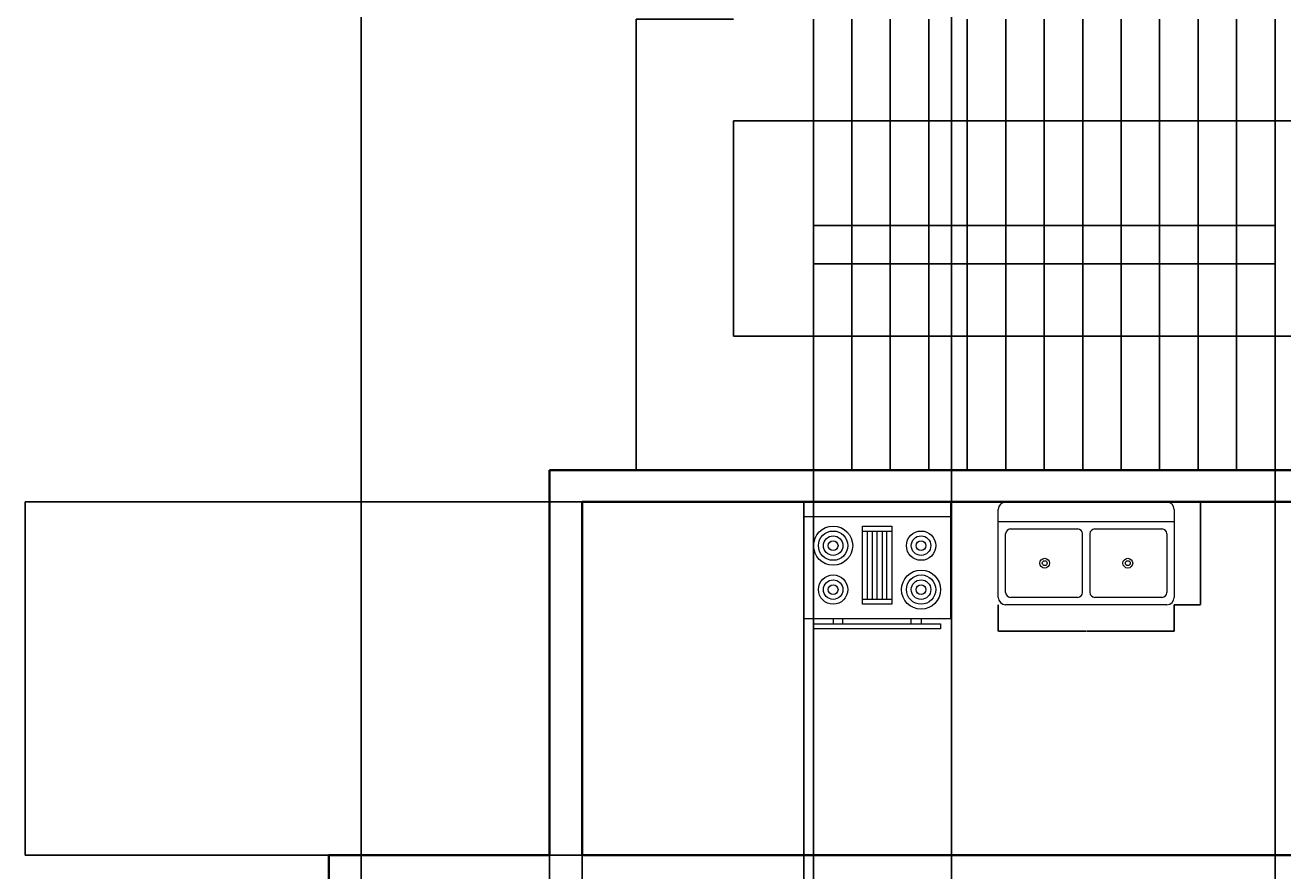
# Model space of a CAD drawing. Units: millimetres. Extents: x 31 to 27050, y -916 to 32407.
# Tile 2 of 7: x 31 to 6569, y 12384 to 16782. Entities that reach past the tile are written whole.
import ezdxf

# ---------------------------------------------------------------- set-up
doc = ezdxf.new("R2010")
doc.units = ezdxf.units.MM
for name, color, linetype, lineweight in [('A-ANNO-DIMS', 2, 'Continuous', 18), ('A-EQPM', 8, 'Continuous', 18), ('A-FLOR-FIXT', 9, 'Continuous', 18), ('A-FLOR-STRS', 7, 'Continuous', 25), ('A-WALL', 7, 'Continuous', 35)]:
    doc.layers.add(name, color=color, linetype=linetype, lineweight=lineweight)
doc.styles.get("Standard").update_dxf_attribs({"font": 'arial.ttf'})
doc.dimstyles.get("Standard").update_dxf_attribs({"dimtxt": 0.18, "dimasz": 0.18, "dimexe": 0.18, "dimexo": 0.0625, "dimgap": 0.09, "dimtad": 0, "dimtih": 1, "dimtoh": 1, "dimdec": 4, "dimzin": 0, "dimdsep": 46, "dimtxsty": 'Standard', "dimcen": 0.09, "dimadec": 0, "dimazin": 0, "dimtfac": 1, "dimtdec": 4, "dimtofl": 0, "dimtmove": 0, "dimatfit": 3, "dimfxl": 1, "dimtolj": 1, "dimtzin": 0, "dimarcsym": 0})

# ---------------------------------------------------------------- blocks, each defined once
blk = doc.blocks.new('Range-Oven - 30 in top')
for p, q in [((0, -3), (30, -3)), ((12, -6), (18, -6)), ((13, -19.999996), (13, -6)), ((14, -6), (14, -19.999996)), ((15, -19.999996), (15, -6)), ((16, -6), (16, -19.999996)), ((17, -19.999996), (17, -6)), ((18, -19.999996), (12, -19.999996)), ((6.000000000000003, -23.99999600000001), (6.000000000000003, -24.999996)), ((8.000000000000004, -24.999996), (8.000000000000004, -23.99999600000001)), ((22.00000000000001, -24.999996), (22.00000000000001, -23.99999600000001)), ((24, -23.99999600000001), (24, -24.999996))]:
    blk.add_line(p, q)
for points in [[(0, -23.99999600000001), (0, 0), (30, 0), (30, -23.99999600000001)], [(12, -20.999996), (12, -5), (18, -5), (18, -20.999996)], [(2.000000000000003, -25.999996), (2.000000000000003, -24.999996), (28.00000000000001, -24.999996), (28.00000000000001, -25.999996)]]:
    blk.add_lwpolyline(points, close=True)
for centre, radius in [((6.000000000000003, -9.0000002), 4), ((6.000000000000003, -9.0000002), 3), ((6.000000000000003, -9.0000002), 2), ((24, -9.0000002), 3), ((24, -9.0000002), 2), ((6.000000000000003, -9.0000002), 1), ((24, -9.0000002), 1), ((6.000000000000003, -18), 3), ((24, -18), 4), ((24, -18), 3), ((6.000000000000003, -18), 2), ((6.000000000000003, -18), 1), ((24, -18), 2), ((24, -18), 1)]:
    blk.add_circle(centre, radius)
blk = doc.blocks.new('Sink-double - 36 in top')
for p, q in [((-18, -4), (18, -4)), ((-0.75, -18.5), (-0.75, -6.5)), ((0.75, -6.5), (0.75, -18.5))]:
    blk.add_line(p, q)
for points in [[(-16.5, 0), (16.5, 0)], [(-18, -19.5), (-18, -1.5)], [(18, -1.5), (18, -19.5)], [(-16.5, -18.5), (-16.5, -6.5)], [(-15.5, -5.5), (-1.75, -5.5)], [(1.75, -5.5), (15.5, -5.5)], [(16.5, -6.5), (16.5, -18.5)], [(-1.75, -19.5), (-15.5, -19.5)], [(15.5, -19.5), (1.75, -19.5)], [(16.5, -21), (-16.5, -21)]]:
    blk.add_lwpolyline(points)
for centre, radius in [((-8.5, -12.5), 1), ((-8.5, -12.5), 0.5), ((8.5, -12.5), 1), ((8.5, -12.5), 0.5)]:
    blk.add_circle(centre, radius)
for centre, radius, start, end in [((-16.5, -1.5), 1.5, 90, 180), ((16.5, -1.5), 1.5, 0, 90), ((-15.5, -6.5), 1, 90, 180), ((-1.75, -6.5), 1, 0, 90), ((1.75, -6.5), 1, 90, 180), ((15.5, -6.5), 1, 0, 90), ((-16.5, -19.5), 1.5, 180, 270), ((-15.5, -18.5), 1, 180, 270), ((-1.75, -18.5), 1, 270, 0), ((1.75, -18.5), 1, 180, 270), ((15.5, -18.5), 1, 270, 0), ((16.5, -19.5), 1.5, 270, 0)]:
    blk.add_arc(centre, radius, start, end)
blk = doc.blocks.new('STAIR-RETURN-2400')
for p, q in [((9.095e-13, 2345.636859649549), (9.095e-13, -1.819e-12)), ((200.0000000000009, 2345.636859649549), (200.0000000000009, -1.819e-12)), ((400.0000000000008, 2345.636859649549), (400.0000000000008, -1.819e-12)), ((600.0000000000008, 2345.636859649549), (600.0000000000008, -1.819e-12)), ((800.0000000000008, 2345.636859649552), (800.0000000000008, 1.819e-12)), ((1000.000000000001, 2345.636859649556), (1000.000000000001, 5.457e-12)), ((1200.000000000001, 2345.636859649556), (1200.000000000001, 5.457e-12)), ((1400.000000000001, 2345.636859649556), (1400.000000000001, 5.457e-12)), ((1600.000000000001, 2345.636859649559), (1600.000000000001, 9.0949e-12)), ((1800.000000000001, 2345.636859649559), (1800.000000000001, 9.0949e-12)), ((2000.000000000001, 2345.636859649559), (2000.000000000001, 9.0949e-12)), ((2200.000000000001, 2345.636859649563), (2200.000000000001, 1.27329e-11)), ((2400.000000000001, 2345.636859649563), (2400.000000000001, 1.27329e-11)), ((-415.9249645337103, 697.4958917418807), (-415.9249645337103, 1817.654410237617)), ((-415.9249645337103, 1817.654410237617), (2588.331988211024, 1817.654410237617)), ((9.095e-13, 1172.818429824772), (9.095e-13, 1272.818429824772)), ((9.095e-13, 1272.818429824772), (2400.000000000001, 1272.818429824774)), ((2400.000000000001, 1272.818429824774), (2400.000000000001, 1072.818429824774)), ((2400.000000000001, 1072.818429824774), (9.095e-13, 1072.818429824774)), ((2597.09055342863, 697.4958917418807), (-415.9249645337103, 697.4958917418807))]:
    blk.add_line(p, q)
blk.add_lwpolyline([(2948.607295106225, 1817.654410237617), (2588.331988211024, 2025.65945565594), (2588.331988211024, 1609.649364819299)], close=True)
blk = doc.blocks.new('*D32')
at = {"layer": 'A-ANNO-DIMS', "color": 0, "lineweight": -2, "transparency": 16777216}
for p, q in [((5090.080722250743, 13767.9627795477), (5090.080722250743, 13630.6852795477)), ((6004.480722250742, 13767.9627795477), (6004.480722250742, 13630.6852795477)), ((5090.260722250743, 13630.8652795477), (5545.806834119774, 13630.8652795477)), ((6004.300722250742, 13630.8652795477), (5548.754610381712, 13630.8652795477))]:
    blk.add_line(p, q, dxfattribs=at)
at = {"layer": 'A-ANNO-DIMS', "color": 0, "transparency": 16777216}
for points in [[(5090.260722250743, 13630.8952795477), (5090.260722250743, 13630.8352795477), (5090.080722250743, 13630.8652795477)], [(6004.300722250742, 13630.8952795477), (6004.300722250742, 13630.8352795477), (6004.480722250742, 13630.8652795477)]]:
    blk.add_solid(points, dxfattribs=at)
at = {"layer": 'Defpoints', "color": 0, "transparency": 16777216}
for p in [(5090.080722250743, 13768.0252795477), (6004.480722250742, 13768.0252795477), (6004.480722250742, 13630.8652795477)]:
    blk.add_point(p, dxfattribs=at)
at = {"layer": 'A-ANNO-DIMS', "color": 0, "transparency": 16777216, "insert": (5547.280722250743, 13630.8652795477), "char_height": 0.18, "attachment_point": 5}
blk.add_mtext('\\A1;DOUBLE SINK 914 TYP.', dxfattribs=at)
blk = doc.blocks.new('*D33')
at = {"layer": 'A-ANNO-DIMS', "color": 0, "lineweight": -2, "transparency": 16777216}
for p, q in [((6004.543222250744, 14301.42527954771), (6141.820722250746, 14301.42527954771)), ((6141.640722250746, 14301.2452795477), (6141.640722250746, 14034.90724407704)), ((6141.640722250746, 13768.20527954771), (6141.640722250746, 14034.54331501838)), ((6004.543222250744, 13768.02527954771), (6141.820722250746, 13768.02527954771))]:
    blk.add_line(p, q, dxfattribs=at)
at = {"layer": 'A-ANNO-DIMS', "color": 0, "transparency": 16777216}
for points in [[(6141.610722250746, 14301.2452795477), (6141.670722250745, 14301.2452795477), (6141.640722250746, 14301.42527954771)], [(6141.610722250746, 13768.20527954771), (6141.670722250745, 13768.20527954771), (6141.640722250746, 13768.02527954771)]]:
    blk.add_solid(points, dxfattribs=at)
at = {"layer": 'Defpoints', "color": 0, "transparency": 16777216}
for p in [(6004.480722250744, 14301.42527954771), (6141.640722250746, 14301.42527954771), (6004.480722250744, 13768.02527954771)]:
    blk.add_point(p, dxfattribs=at)
at = {"layer": 'A-ANNO-DIMS', "color": 0, "transparency": 16777216, "insert": (6141.640722250748, 14034.7252795477), "char_height": 0.18, "attachment_point": 5}
blk.add_mtext('\\A1;533 TYP.', dxfattribs=at)
blk = doc.blocks.new('*D41')
at = {"layer": 'A-ANNO-DIMS', "color": 0, "lineweight": -2, "transparency": 16777216}
for p, q in [((3712.606591999184, 16813.06179635637), (3207.809253053195, 16813.06179635637)), ((3207.989253053195, 16812.88179635637), (3207.989253053195, 15640.42533106092)), ((3207.989253053195, 14467.60493670681), (3207.989253053195, 15640.06140200226)), ((3712.606591999184, 14467.4249367068), (3207.809253053195, 14467.4249367068))]:
    blk.add_line(p, q, dxfattribs=at)
at = {"layer": 'A-ANNO-DIMS', "color": 0, "transparency": 16777216}
for points in [[(3207.959253053195, 16812.88179635637), (3208.019253053195, 16812.88179635637), (3207.989253053195, 16813.06179635637)], [(3207.959253053195, 14467.60493670681), (3208.019253053195, 14467.60493670681), (3207.989253053195, 14467.4249367068)]]:
    blk.add_solid(points, dxfattribs=at)
at = {"layer": 'Defpoints', "color": 0, "transparency": 16777216}
for p in [(3207.989253053195, 16813.06179635637), (3712.669091999184, 16813.06179635637), (3712.669091999184, 14467.4249367068)]:
    blk.add_point(p, dxfattribs=at)
at = {"layer": 'A-ANNO-DIMS', "color": 0, "transparency": 16777216, "insert": (3207.989253053199, 15640.24336653158), "char_height": 0.18, "attachment_point": 5}
blk.add_mtext('\\A1;2346 TYP.', dxfattribs=at)
blk = doc.blocks.new('*D56')
at = {"layer": 'A-ANNO-DIMS', "color": 0, "lineweight": -2, "transparency": 16777216}
for p, q in [((2925.628986000001, 14303.541814), (30.84199700000001, 14303.541814)), ((31.02199699999983, 14303.36181400001), (31.02199700000003, 13384.82470702934)), ((31.02199700000023, 12465.923671), (31.02199700000003, 13384.46077797067)), ((2925.628986000001, 12465.74367100001), (30.84199700000042, 12465.74367100001))]:
    blk.add_line(p, q, dxfattribs=at)
at = {"layer": 'A-ANNO-DIMS', "color": 0, "transparency": 16777216}
for points in [[(30.99199699999982, 14303.36181400001), (31.05199699999983, 14303.36181400001), (31.02199699999983, 14303.541814)], [(30.99199700000023, 12465.923671), (31.05199700000023, 12465.923671), (31.02199700000023, 12465.74367100001)]]:
    blk.add_solid(points, dxfattribs=at)
at = {"layer": 'Defpoints', "color": 0, "transparency": 16777216}
for p in [(31.02199699999983, 14303.541814), (2925.691486000001, 14303.541814), (2925.691486000001, 12465.74367100001)]:
    blk.add_point(p, dxfattribs=at)
at = {"layer": 'A-ANNO-DIMS', "color": 0, "transparency": 16777216, "insert": (31.02199700000382, 13384.6427425), "char_height": 0.18, "attachment_point": 5}
blk.add_mtext('\\A1;1837.8', dxfattribs=at)
blk = doc.blocks.new('*D61')
at = {"layer": 'A-ANNO-DIMS', "color": 0, "lineweight": -2, "transparency": 16777216}
for p, q in [((1778.372648, 7250.606205), (1778.372648000001, 32406.711259)), ((1778.552648000001, 32406.531259), (3312.109331318556, 32406.531259)), ((4846.592413000001, 32406.531259), (3313.035729681448, 32406.531259)), ((4846.772413, 7250.606205), (4846.772413000001, 32406.711259))]:
    blk.add_line(p, q, dxfattribs=at)
at = {"layer": 'A-ANNO-DIMS', "color": 0, "transparency": 16777216}
for points in [[(1778.552648000001, 32406.561259), (1778.552648000001, 32406.501259), (1778.372648000001, 32406.531259)], [(4846.592413000001, 32406.561259), (4846.592413000001, 32406.501259), (4846.772413000001, 32406.531259)]]:
    blk.add_solid(points, dxfattribs=at)
at = {"layer": 'Defpoints', "color": 0, "transparency": 16777216}
for p in [(4846.772413000001, 32406.531259), (1778.372648, 7250.543705), (4846.772413, 7250.543705)]:
    blk.add_point(p, dxfattribs=at)
at = {"layer": 'A-ANNO-DIMS', "color": 0, "transparency": 16777216, "insert": (3312.572530500002, 32406.531259), "char_height": 0.18, "attachment_point": 5}
blk.add_mtext('\\A1;3068.4', dxfattribs=at)
blk = doc.blocks.new('*D69')
at = {"layer": 'A-ANNO-DIMS', "color": 0, "lineweight": -2, "transparency": 16777216}
for p, q in [((2757.340836, 14467.362437), (2757.340835999999, -915.5318640000004)), ((4128.594056999999, 14467.362437), (4128.594056999999, -915.5318640000004)), ((2757.520835999999, -915.3518639999999), (3442.512289610504, -915.3518639999999)), ((4128.414056999999, -915.3518639999999), (3443.422603389495, -915.3518639999999))]:
    blk.add_line(p, q, dxfattribs=at)
at = {"layer": 'A-ANNO-DIMS', "color": 0, "transparency": 16777216}
for points in [[(2757.520835999999, -915.321864), (2757.520835999999, -915.381864), (2757.340835999999, -915.3518639999999)], [(4128.414056999999, -915.321864), (4128.414056999999, -915.381864), (4128.594056999999, -915.3518639999999)]]:
    blk.add_solid(points, dxfattribs=at)
at = {"layer": 'Defpoints', "color": 0, "transparency": 16777216}
for p in [(2757.340836, 14467.424937), (4128.594056999999, 14467.424937), (4128.594056999999, -915.3518639999999)]:
    blk.add_point(p, dxfattribs=at)
at = {"layer": 'A-ANNO-DIMS', "color": 0, "transparency": 16777216, "insert": (3442.967446499999, -915.3518639999999), "char_height": 0.18, "attachment_point": 5}
blk.add_mtext('\\A1;1371.3', dxfattribs=at)
blk = doc.blocks.new('*D70')
at = {"layer": 'A-ANNO-DIMS', "color": 0, "lineweight": -2, "transparency": 16777216}
for p, q in [((4128.594056999999, 14467.362437), (4128.594056999999, -915.5318640000004)), ((6528.594057000001, 14467.362437), (6528.594056999999, -915.5318640000004)), ((4128.774057, -915.3518639999999), (5328.234056999999, -915.3518639999999)), ((6528.414056999999, -915.3518639999999), (5328.954056999999, -915.3518639999999))]:
    blk.add_line(p, q, dxfattribs=at)
at = {"layer": 'A-ANNO-DIMS', "color": 0, "transparency": 16777216}
for points in [[(4128.774057, -915.321864), (4128.774057, -915.381864), (4128.594056999999, -915.3518639999999)], [(6528.414056999999, -915.321864), (6528.414056999999, -915.381864), (6528.594056999999, -915.3518639999999)]]:
    blk.add_solid(points, dxfattribs=at)
at = {"layer": 'Defpoints', "color": 0, "transparency": 16777216}
for p in [(4128.594056999999, 14467.424937), (6528.594057000001, 14467.424937), (6528.594056999999, -915.3518639999999)]:
    blk.add_point(p, dxfattribs=at)
at = {"layer": 'A-ANNO-DIMS', "color": 0, "transparency": 16777216, "insert": (5328.594057, -915.3518639999999), "char_height": 0.18, "attachment_point": 5}
blk.add_mtext('\\A1;2400', dxfattribs=at)
blk = doc.blocks.new('*D93')
at = {"layer": 'A-ANNO-DIMS', "color": 0, "lineweight": -2, "transparency": 16777216}
for p, q in [((2925.691486, 14303.479314), (2925.691486, -915.5318640000004)), ((4078.94748, 14303.479314), (4078.947479999999, -915.5318640000004)), ((2925.871485999999, -915.3518639999999), (3501.864326110504, -915.3518639999999)), ((4078.767479999998, -915.3518639999999), (3502.774639889495, -915.3518639999999))]:
    blk.add_line(p, q, dxfattribs=at)
at = {"layer": 'A-ANNO-DIMS', "color": 0, "transparency": 16777216}
for points in [[(2925.871485999999, -915.321864), (2925.871485999999, -915.381864), (2925.691486, -915.3518639999999)], [(4078.767479999998, -915.321864), (4078.767479999998, -915.381864), (4078.947479999999, -915.3518639999999)]]:
    blk.add_solid(points, dxfattribs=at)
at = {"layer": 'Defpoints', "color": 0, "transparency": 16777216}
for p in [(2925.691486, 14303.541814), (4078.94748, 14303.541814), (4078.947479999999, -915.3518639999999)]:
    blk.add_point(p, dxfattribs=at)
at = {"layer": 'A-ANNO-DIMS', "color": 0, "transparency": 16777216, "insert": (3502.319482999999, -915.3518639999999), "char_height": 0.18, "attachment_point": 5}
blk.add_mtext('\\A1;1153.3', dxfattribs=at)

msp = doc.modelspace()

# ---------------------------------------------------------------- linework, layer by layer
at = {"layer": 'A-WALL'}
for p, q in [((2757.34083568836, 14467.4249367068), (9517.798935037174, 14467.4249367068)), ((2757.340835688359, 14467.4249367068), (2757.340835688359, 14303.54181440175)), ((2757.340835688364, 12465.74367114627), (2757.340835688365, 14303.54181440175)), ((2925.691486399059, 12465.74367114627), (2925.691486399059, 14303.54181440175)), ((2925.691486399059, 14303.54181440175), (9513.331406631527, 14303.54181440175)), ((1610.021997114469, 744.3803777755929), (1610.021997114469, 12465.74367114627)), ((1778.372647825162, 12465.74367114627), (1610.021997114468, 12465.74367114627)), ((2757.340835688364, 12465.74367114627), (1778.372647825163, 12465.74367114627)), ((8211.090788713413, 12465.74367114626), (2925.691486399059, 12465.74367114627))]:
    msp.add_line(p, q, dxfattribs=at)

# ---------------------------------------------------------------- block references
at = {"layer": 'A-EQPM', "xscale": 25.4, "yscale": 25.4, "zscale": 25.4}
msp.add_blockref('Range-Oven - 30 in top', (4078.947479641334, 14303.54181440175), dxfattribs=at)
at = {"layer": 'A-FLOR-FIXT', "xscale": 25.4, "yscale": 25.4, "zscale": 25.4}
msp.add_blockref('Sink-double - 36 in top', (5547.280722250743, 14301.4252795477), dxfattribs=at)
at = {"layer": 'A-FLOR-STRS'}
msp.add_blockref('STAIR-RETURN-2400', (4128.594056532892, 14467.4249367068), dxfattribs=at)

# ---------------------------------------------------------------- dimensions: what is measured, and where the dimension line sits
at = {"layer": 'A-ANNO-DIMS'}
for base, p1, p2, override, picture, middle in [((4846.772413000001, 32406.531259), (1778.372648, 7250.543705), (4846.772413, 7250.543705), {"dimdec": 1, "dimlfac": 1, "dimrnd": 0, "dimzin": 0, "dimdsep": 46, "dimlunit": 2}, '*D61', (3312.572530500002, 32406.531259)), ((4128.594056999999, -915.3518639999999), (2757.340836, 14467.424937), (4128.594056999999, 14467.424937), {"dimdec": 1, "dimlfac": 1, "dimrnd": 0, "dimzin": 0, "dimdsep": 46, "dimlunit": 2}, '*D69', (3442.967446499999, -915.3518639999999)), ((6528.594056999999, -915.3518639999999), (4128.594056999999, 14467.424937), (6528.594057000001, 14467.424937), {"dimdec": 0, "dimlfac": 1, "dimrnd": 0, "dimzin": 0, "dimdsep": 46, "dimlunit": 2}, '*D70', (5328.594057, -915.3518639999999)), ((4078.947479999999, -915.3518639999999), (2925.691486, 14303.541814), (4078.94748, 14303.541814), {"dimdec": 1, "dimlfac": 1, "dimrnd": 0, "dimzin": 0, "dimdsep": 46, "dimlunit": 2}, '*D93', (3502.319482999999, -915.3518639999999))]:
    dim = msp.add_linear_dim(base=base, p1=p1, p2=p2, dimstyle='Standard', override=override, dxfattribs=at)
    dim.commit()
    dim.dimension.update_dxf_attribs({"geometry": picture, "text_midpoint": middle})
for base, p1, p2, picture, middle in [((3207.989253053195, 16813.06179635637), (3712.669091999182, 14467.4249367068), (3712.669091999182, 16813.06179635636), '*D41', (3207.989253053199, 15640.24336653158)), ((6141.640722250746, 14301.42527954771), (6004.480722250742, 13768.0252795477), (6004.480722250742, 14301.4252795477), '*D33', (6141.640722250748, 14034.7252795477))]:
    dim = msp.add_linear_dim(base=base, p1=p1, p2=p2, angle=90, text='<> TYP.', dimstyle='Standard', override={"dimdec": 0, "dimlfac": 1, "dimrnd": 0, "dimzin": 0, "dimdsep": 46, "dimlunit": 2}, dxfattribs=at)
    dim.commit()
    dim.dimension.update_dxf_attribs({"geometry": picture, "text_midpoint": middle})
dim = msp.add_linear_dim(base=(31.02199699999983, 14303.541814), p1=(2925.691486, 12465.743671), p2=(2925.691486, 14303.541814), angle=90, dimstyle='Standard', override={"dimdec": 1, "dimlfac": 1, "dimrnd": 0, "dimzin": 0, "dimdsep": 46, "dimlunit": 2}, dxfattribs=at)
dim.commit()
dim.dimension.update_dxf_attribs({"geometry": '*D56', "text_midpoint": (31.02199700000382, 13384.6427425)})
dim = msp.add_linear_dim(base=(6004.480722250742, 13630.8652795477), p1=(5090.080722250743, 13768.0252795477), p2=(6004.480722250742, 13768.0252795477), text='DOUBLE SINK <> TYP.', dimstyle='Standard', override={"dimdec": 0, "dimlfac": 1, "dimrnd": 0, "dimzin": 0, "dimdsep": 46, "dimlunit": 2}, dxfattribs=at)
dim.commit()
dim.dimension.update_dxf_attribs({"geometry": '*D32', "text_midpoint": (5547.280722250743, 13630.8652795477)})

doc.saveas('drawing.dxf')
